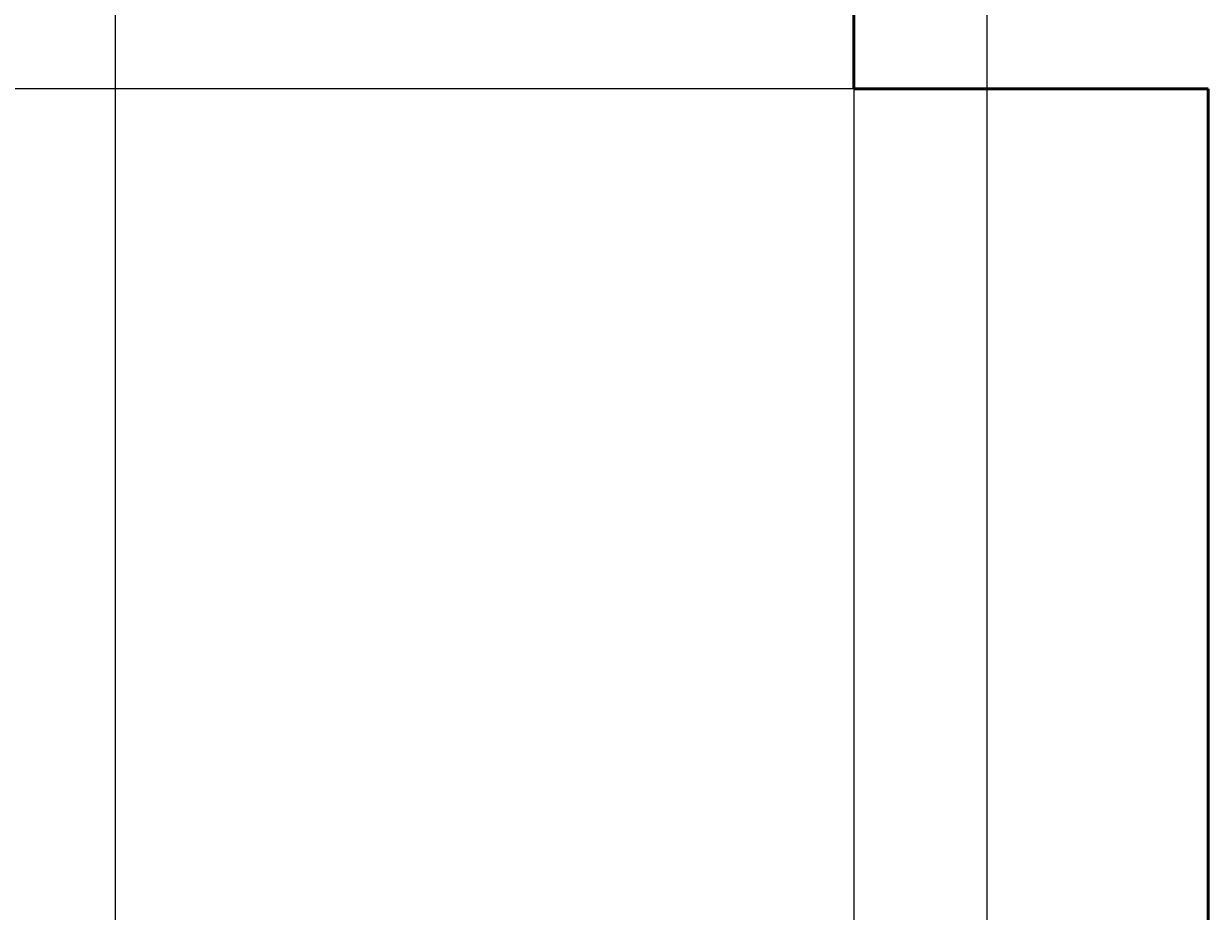
# Model space of a CAD drawing. Units: inches. Extents: x 5375 to 6084, y 16106 to 17259.
# Tile 20 of 32: x 5464 to 5545, y 16812 to 16872. Entities that reach past the tile are written whole.
import ezdxf

# ---------------------------------------------------------------- set-up
doc = ezdxf.new("R2010")
doc.units = ezdxf.units.IN
doc.layers.add('A-ANNO-DIMS', color=2, linetype='Continuous', lineweight=18)
doc.layers.add('WALL', color=6, linetype='Continuous', lineweight=50)
doc.styles.get("Standard").update_dxf_attribs({"font": 'arial.ttf'})
doc.dimstyles.get("Standard").update_dxf_attribs({"dimtxt": 0.18, "dimasz": 0.18, "dimexe": 0.18, "dimexo": 0.0625, "dimgap": 0.09, "dimtad": 0, "dimtih": 1, "dimtoh": 1, "dimdec": 4, "dimzin": 0, "dimdsep": 46, "dimtxsty": 'Standard', "dimcen": 0.09, "dimadec": 0, "dimazin": 0, "dimtfac": 1, "dimtdec": 4, "dimtofl": 0, "dimtmove": 0, "dimatfit": 3, "dimfxl": 1, "dimtolj": 1, "dimtzin": 0, "dimarcsym": 0})

# ---------------------------------------------------------------- blocks, each defined once
blk = doc.blocks.new('*D36')
at = {"layer": 'A-ANNO-DIMS', "color": 0, "lineweight": -2, "transparency": 16777216}
for p, q in [((5544.557, 16867.579), (5375.562, 16867.579)), ((5375.742, 16867.399), (5375.742, 16783.761)), ((5375.742, 16699.759), (5375.742, 16783.397)), ((5544.557, 16699.579), (5375.562, 16699.579))]:
    blk.add_line(p, q, dxfattribs=at)
at = {"layer": 'A-ANNO-DIMS', "color": 0, "transparency": 16777216}
for points in [[(5375.712, 16867.399), (5375.772, 16867.399), (5375.742, 16867.579)], [(5375.712, 16699.759), (5375.772, 16699.759), (5375.742, 16699.579)]]:
    blk.add_solid(points, dxfattribs=at)
at = {"layer": 'Defpoints', "color": 0, "transparency": 16777216}
for p in [(5375.742, 16867.579), (5544.62, 16867.579), (5544.62, 16699.579)]:
    blk.add_point(p, dxfattribs=at)
at = {"layer": 'A-ANNO-DIMS', "color": 0, "transparency": 16777216, "insert": (5375.742, 16783.579), "char_height": 0.18, "attachment_point": 5}
blk.add_mtext('\\A1;168', dxfattribs=at)
blk = doc.blocks.new('*D37')
at = {"layer": 'A-ANNO-DIMS', "color": 0, "lineweight": -2, "transparency": 16777216}
for p, q in [((5520.557, 17206.579), (5375.562, 17206.579)), ((5375.742, 17206.399), (5375.742, 17037.261)), ((5375.742, 16867.759), (5375.742, 17036.897)), ((5520.557, 16867.579), (5375.562, 16867.579))]:
    blk.add_line(p, q, dxfattribs=at)
at = {"layer": 'A-ANNO-DIMS', "color": 0, "transparency": 16777216}
for points in [[(5375.712, 17206.399), (5375.772, 17206.399), (5375.742, 17206.579)], [(5375.712, 16867.759), (5375.772, 16867.759), (5375.742, 16867.579)]]:
    blk.add_solid(points, dxfattribs=at)
at = {"layer": 'Defpoints', "color": 0, "transparency": 16777216}
for p in [(5375.742, 17206.579), (5520.62, 17206.579), (5520.62, 16867.579)]:
    blk.add_point(p, dxfattribs=at)
at = {"layer": 'A-ANNO-DIMS', "color": 0, "transparency": 16777216, "insert": (5375.742, 17037.079), "char_height": 0.18, "attachment_point": 5}
blk.add_mtext('\\A1;339', dxfattribs=at)
blk = doc.blocks.new('*D40')
at = {"layer": 'A-ANNO-DIMS', "color": 0, "lineweight": -2, "transparency": 16777216}
for p, q in [((5529.62, 16876.517), (5529.62, 16106.483)), ((5520.62, 16867.517), (5520.62, 16106.483)), ((5520.8, 16106.663), (5524.971, 16106.663)), ((5529.44, 16106.663), (5525.269, 16106.663))]:
    blk.add_line(p, q, dxfattribs=at)
at = {"layer": 'A-ANNO-DIMS', "color": 0, "transparency": 16777216}
for points in [[(5520.8, 16106.693), (5520.8, 16106.633), (5520.62, 16106.663)], [(5529.44, 16106.693), (5529.44, 16106.633), (5529.62, 16106.663)]]:
    blk.add_solid(points, dxfattribs=at)
at = {"layer": 'Defpoints', "color": 0, "transparency": 16777216}
for p in [(5529.62, 16876.579), (5520.62, 16867.579), (5529.62, 16106.663)]:
    blk.add_point(p, dxfattribs=at)
at = {"layer": 'A-ANNO-DIMS', "color": 0, "transparency": 16777216, "insert": (5525.12, 16106.663), "char_height": 0.18, "attachment_point": 5}
blk.add_mtext('\\A1;9', dxfattribs=at)
blk = doc.blocks.new('*D47')
at = {"layer": 'A-ANNO-DIMS', "color": 0, "lineweight": -2, "transparency": 16777216}
for p, q in [((5470.62, 16603.642), (5470.62, 17259.159)), ((5470.8, 17258.979), (5495.401, 17258.979)), ((5520.44, 17258.979), (5495.839, 17258.979)), ((5520.62, 17206.642), (5520.62, 17259.159))]:
    blk.add_line(p, q, dxfattribs=at)
at = {"layer": 'A-ANNO-DIMS', "color": 0, "transparency": 16777216}
for points in [[(5470.8, 17259.009), (5470.8, 17258.949), (5470.62, 17258.979)], [(5520.44, 17259.009), (5520.44, 17258.949), (5520.62, 17258.979)]]:
    blk.add_solid(points, dxfattribs=at)
at = {"layer": 'Defpoints', "color": 0, "transparency": 16777216}
for p in [(5520.62, 17258.979), (5520.62, 17206.579), (5470.62, 16603.579)]:
    blk.add_point(p, dxfattribs=at)
at = {"layer": 'A-ANNO-DIMS', "color": 0, "transparency": 16777216, "insert": (5495.62, 17258.979), "char_height": 0.18, "attachment_point": 5}
blk.add_mtext('\\A1;50', dxfattribs=at)

msp = doc.modelspace()

# ---------------------------------------------------------------- linework, layer by layer
at = {"layer": 'WALL'}
for p, q in [((5520.6199, 17206.5793), (5520.6199, 16867.5793)), ((5520.6199, 16867.5793), (5544.6199, 16867.5793)), ((5544.6199, 16867.5793), (5544.6199, 16699.5793))]:
    msp.add_line(p, q, dxfattribs=at)

# ---------------------------------------------------------------- dimensions: what is measured, and where the dimension line sits
at = {"layer": 'A-ANNO-DIMS'}
for base, p1, p2, picture, middle in [((5520.6199, 17258.9793), (5470.6199, 16603.5793), (5520.6199, 17206.5793), '*D47', (5495.6199, 17258.9793)), ((5529.6199, 16106.6631), (5520.6199, 16867.5793), (5529.6199, 16876.5793), '*D40', (5525.1199, 16106.6631))]:
    dim = msp.add_linear_dim(base=base, p1=p1, p2=p2, dimstyle='Standard', override={"dimdec": 0, "dimlfac": 1, "dimrnd": 0, "dimzin": 0, "dimdsep": 46, "dimlunit": 2}, dxfattribs=at)
    dim.commit()
    dim.dimension.update_dxf_attribs({"geometry": picture, "text_midpoint": middle})
for base, p1, p2, picture, middle in [((5375.7423, 17206.5793), (5520.6199, 16867.5793), (5520.6199, 17206.5793), '*D37', (5375.7423, 17037.0793)), ((5375.7423, 16867.5793), (5544.6199, 16699.5793), (5544.6199, 16867.5793), '*D36', (5375.7423, 16783.5793))]:
    dim = msp.add_linear_dim(base=base, p1=p1, p2=p2, angle=90, dimstyle='Standard', override={"dimdec": 0, "dimlfac": 1, "dimrnd": 0, "dimzin": 0, "dimdsep": 46, "dimlunit": 2}, dxfattribs=at)
    dim.commit()
    dim.dimension.update_dxf_attribs({"geometry": picture, "text_midpoint": middle})

doc.saveas('drawing.dxf')
